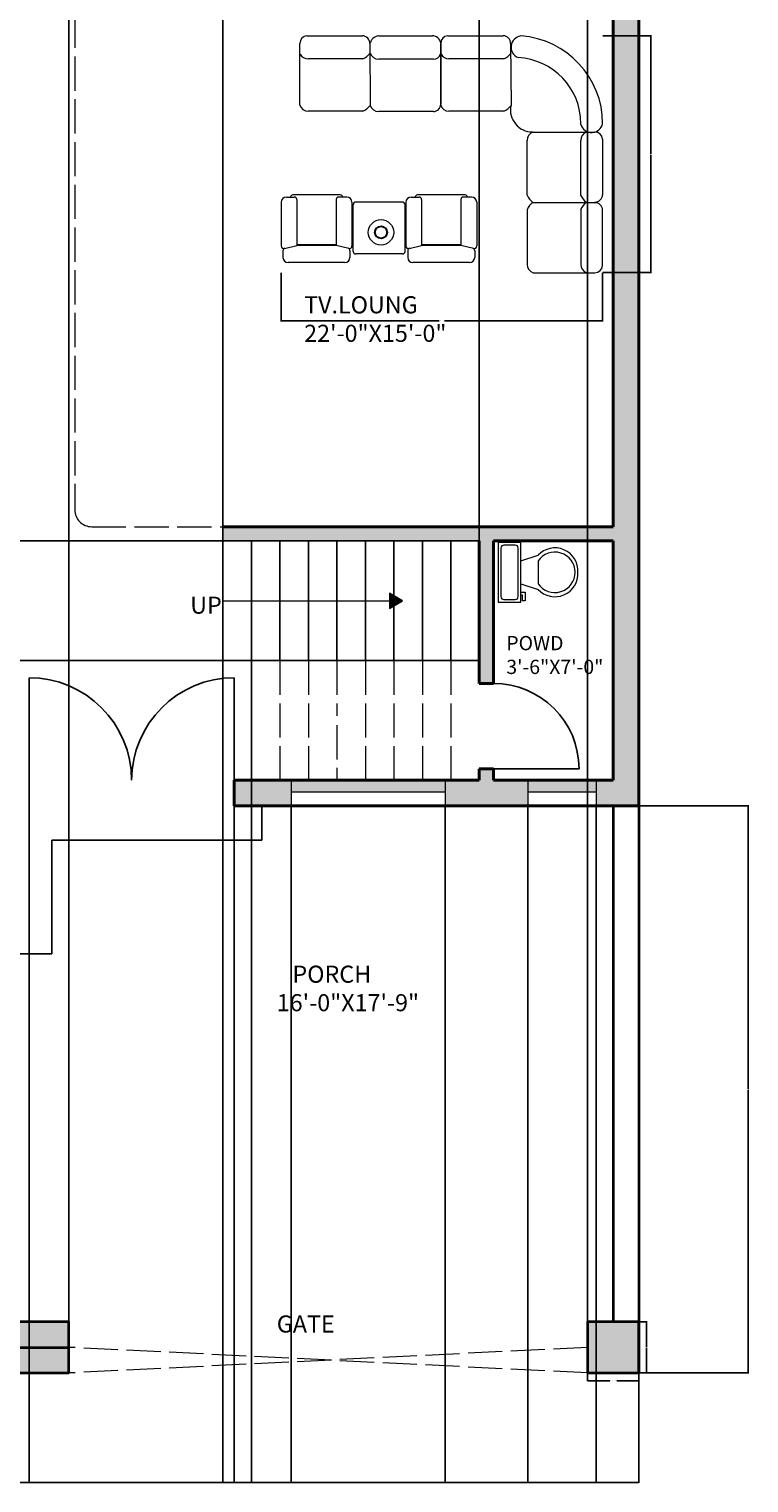
# Model space of a CAD drawing. Units: inches. Extents: x 2985 to 3527, y 3685 to 4528.
# Tile 2 of 5: x 3274 to 3527, y 3685 to 4195. Entities that reach past the tile are written whole.
import ezdxf

# ---------------------------------------------------------------- set-up
doc = ezdxf.new("R2010")
doc.units = ezdxf.units.IN
doc.linetypes.add('ACAD_ISO02W100', pattern=[15, 12, -3])
for name, color, linetype, lineweight in [('A-ANNO-DIMS', 2, 'Continuous', 18), ('A-ANNO-SYMB', 7, 'Continuous', 18), ('A-ANNO-TEXT', 7, 'Continuous', 18), ('A-AREA-IDEN', 7, 'Continuous', 25), ('A-FLOR-EDGE', 7, 'Continuous', 25), ('A-FLOR-FIXT', 9, 'Continuous', 18), ('A-FLOR-STRS', 7, 'Continuous', 25), ('A-FLOR-STRS-OVHD', 7, 'ACAD_ISO02W100', 18), ('A-FURN', 8, 'Continuous', 18), ('A-GLAZ', 4, 'Continuous', 18), ('A-SITE-GATE', 4, 'ACAD_ISO02W100', 18), ('A-SITE-WALL', 7, 'Continuous', 35), ('A-WALL', 7, 'Continuous', 40), ('A-WALL-OVHD', 7, 'ACAD_ISO02W100', 18), ('A-WALL-PATT', 8, 'Continuous', 13), ('door', 4, 'Continuous', 25)]:
    doc.layers.add(name, color=color, linetype=linetype, lineweight=lineweight)
doc.layers.add('A-GLAZ-PATT', color=241, linetype='Continuous', lineweight=13, true_color=0xf7abae)
doc.styles.get("Standard").update_dxf_attribs({"font": 'arial.ttf'})
doc.dimstyles.get("Standard").update_dxf_attribs({"dimtxt": 0.18, "dimasz": 0.18, "dimexe": 0.18, "dimexo": 0.0625, "dimgap": 0.09, "dimtad": 0, "dimtih": 1, "dimtoh": 1, "dimdec": 4, "dimzin": 0, "dimdsep": 46, "dimtxsty": 'Standard', "dimcen": 0.09, "dimadec": 0, "dimazin": 0, "dimtfac": 1, "dimtdec": 4, "dimtofl": 0, "dimtmove": 0, "dimatfit": 3, "dimfxl": 1, "dimtolj": 1, "dimtzin": 0, "dimarcsym": 0})

# ---------------------------------------------------------------- blocks, each defined once
blk = doc.blocks.new('*U7')
for p, q in [((9.5, -6), (9.5, -2)), ((-10, -8.5), (-8, -8.5)), ((-10, -9.5), (-10, -8.5)), ((-7, -9.5), (-10, -9.5)), ((-8, -8.5), (-8, -8)), ((-7, -8), (-7, -9.5)), ((-4, -8), (-6, -14)), ((4, -8), (6, -14)), ((4, -14), (-4, -14))]:
    blk.add_line(p, q)
blk.add_lwpolyline([(10.5, -8), (10.5, 0), (-10.5, 0), (-10.5, -8)], close=True)
for points in [[(-9.5, -2), (-9.5, -6)], [(8.5, -1), (-8.5, -1)], [(-8.5, -7), (8.5, -7)]]:
    blk.add_lwpolyline(points)
for centre, radius, start, end in [((-8.625, -1.875), 0.8839, 81.8699, 188.1301), ((8.625, -1.875), 0.8839, 351.8699, 98.1301), ((-8.625, -6.125), 0.8839, 171.869898, 278.1301), ((8.625, -6.125), 0.8839, 261.8699, 8.1301), ((-0.4772, -19.9188), 8.0953, 133.01722, 273.38), ((0.0374, -19.8731), 7.127, 124.50543, 269.7), ((-0.0373, -19.8731), 7.127, 270.3, 55.4946), ((0.4773, -19.9188), 8.0953, 266.62, 46.9828)]:
    blk.add_arc(centre, radius, start, end)
blk = doc.blocks.new('A$C6748376E')
for p, q in [((297, 2742), (941, 2742)), ((1126, 2742), (1751, 2742)), ((1929, 2742), (2572, 2742)), ((216, 1940), (216, 2654)), ((1026, 2654), (1030, 1936)), ((1847, 2661), (1847, 1951)), ((1847, 1940), (1847, 2654)), ((2657, 2654), (2661, 1936)), ((945, 2475), (312, 2475)), ((1289, 2472), (1130, 2472)), ((1762, 2472), (1289, 2472)), ((2576, 2475), (1943, 2475)), ((945, 1870), (312, 1870)), ((1289, 1866), (1130, 1866)), ((1762, 1866), (1289, 1866)), ((2576, 1870), (1943, 1870)), ((3469, 1717), (3469, 1725)), ((2848, 899), (2848, 1532)), ((2918, 1628), (3632, 1628)), ((3468, 899), (3468, 1532)), ((3538, 1628), (3541, 1628)), ((3721, 1546), (3721, 903)), ((60, 876), (151, 876)), ((684, 900), (136, 900)), ((181, 846), (181, 316)), ((637, 846), (637, 316)), ((760, 876), (667, 876)), ((1504, 876), (1596, 876)), ((2129, 900), (1580, 900)), ((1626, 846), (1626, 316)), ((2081, 846), (2081, 316)), ((2204, 876), (2111, 876)), ((0, 816), (0, 309)), ((820, 816), (820, 309)), ((834, 247), (834, 787)), ((1404, 817), (864, 817)), ((1434, 247), (1434, 787)), ((1444, 816), (1444, 309)), ((2264, 816), (2264, 309)), ((2848, 729), (2848, 96)), ((2915, 814), (3632, 818)), ((2915, 814), (3632, 810)), ((3468, 729), (3468, 96)), ((3721, 81), (3721, 725)), ((21, 253), (21, 246)), ((21, 246), (21, 176)), ((37, 280), (181, 316)), ((637, 324), (181, 324)), ((637, 316), (181, 316)), ((783, 280), (637, 316)), ((797, 253), (797, 176)), ((1404, 217), (864, 217)), ((1466, 253), (1466, 246)), ((1466, 246), (1466, 176)), ((1482, 280), (1626, 316)), ((2081, 324), (1626, 324)), ((2081, 316), (1626, 316)), ((2227, 280), (2081, 316)), ((2241, 253), (2241, 176)), ((737, 116), (81, 116)), ((2181, 116), (1526, 116)), ((2918, 0), (3632, 0)), ((3538, 0), (3541, 0))]:
    blk.add_line(p, q)
for radius in [147, 75, 66]:
    blk.add_circle((1156, 467), radius)
for centre, radius, start, end in [((305, 2654), 89.1, 94.9502, 180), ((941, 2657), 85.2, 357.5912, 90), ((1147, 2618), 126, 99.5063, 163.732), ((1751, 2645), 97.5, 9.5558, 90), ((1936, 2654), 89.1, 94.9502, 180), ((2572, 2657), 85.2, 357.5912, 90), ((2793, 2611), 131, 98.1187, 247.4204), ((2704, 1725), 1018, 0.0517, 86.013), ((312, 2576), 101, 205.9257, 270), ((864, 2667), 208, 292.9498, 323.1162), ((1130, 2578), 106, 199.7589, 270), ((1762, 2557), 85, 269.971, 343.2423), ((1943, 2576), 101, 205.9257, 270), ((2495, 2667), 208, 292.9498, 323.1162), ((2704, 1725), 766, 0, 87.0841), ((312, 1971), 101, 197.7112, 270), ((864, 2061), 208, 292.9498, 323.1162), ((1130, 1972), 106, 199.7589, 270), ((1762, 1951), 85, 269.971, 0), ((1943, 1971), 101, 197.7112, 270), ((2495, 2061), 208, 292.9498, 323.1162), ((2909, 1885), 255, 169.3994, 270), ((3594, 1754), 131, 196.7665, 347.5739), ((2949, 1532), 101, 107.7112, 180), ((3569, 1532), 101, 107.7112, 180), ((3632, 1539), 89.1, 4.9502, 90), ((60, 816), 60, 90, 180), ((136, 870), 30, 90, 180), ((151, 846), 30, 0, 90), ((667, 846), 30, 90, 180), ((684, 870), 30, 0, 90), ((760, 816), 60, 0, 90), ((1504, 816), 60, 90, 180), ((1580, 870), 30, 90, 180), ((1596, 846), 30, 0, 90), ((2111, 846), 30, 90, 180), ((2129, 870), 30, 0, 90), ((2204, 816), 60, 0, 90), ((3039, 980), 208, 202.9498, 233.1162), ((3659, 980), 208, 202.9498, 233.1162), ((3636, 903), 85.2, 267.5912, 0), ((864, 787), 30, 90, 180), ((1404, 787), 30, 0, 90), ((3039, 648), 208, 126.8838, 157.0502), ((3659, 648), 208, 126.8838, 157.0502), ((3636, 725), 85.2, 0, 92.4088), ((30, 309), 30, 180, 284.0362), ((51, 253), 30, 104.0362, 180), ((81, 176), 60, 180, 270), ((737, 176), 60, 270, 0), ((767, 253), 30, 0, 75.9638), ((790, 309), 30, 255.9638, 0), ((864, 247), 30, 180, 270), ((1404, 247), 30, 270, 0), ((1474, 309), 30, 180, 284.0362), ((1496, 253), 30, 104.0362, 180), ((1526, 176), 60, 180, 270), ((2181, 176), 60, 270, 0), ((2211, 253), 30, 0, 75.9638), ((2234, 309), 30, 255.9638, 0), ((2949, 96), 101, 180, 252.2888), ((3569, 96), 101, 180, 252.2888), ((3632, 89), 89.1, 270, 355.0498)]:
    blk.add_arc(centre, radius, start, end)
blk = doc.blocks.new('DOOR-SWING-30IN')
blk.add_line((0, 0), (30, 0))
blk.add_arc((0, 0), 30, 0, 90)
blk = doc.blocks.new('DOOR-SWING-36IN')
blk.add_line((0, 0), (0, 36))
blk.add_arc((0, 0), 36, 0, 90)
blk = doc.blocks.new('GATE-PIER-18IN')
h = blk.add_hatch(color=256)
h.dxf.hatch_style = 1
h.paths.add_polyline_path([(18, 0), (18, 18), (0, 18), (0, 0)])
blk.add_lwpolyline([(0, 0), (18, 0), (18, 18), (0, 18)], close=True)
blk = doc.blocks.new('*D30')
at = {"layer": 'A-ANNO-DIMS', "color": 0, "lineweight": -2, "transparency": 16777216}
for p, q in [((3470.33, 3723.31), (3470.33, 3720.49)), ((3470.51, 3720.67), (3478.1, 3720.67)), ((3488.15, 3720.67), (3480.57, 3720.67)), ((3488.33, 3723.31), (3488.33, 3720.49))]:
    blk.add_line(p, q, dxfattribs=at)
at = {"layer": 'A-ANNO-DIMS', "color": 0, "transparency": 16777216}
for points in [[(3470.51, 3720.7), (3470.51, 3720.64), (3470.33, 3720.67)], [(3488.15, 3720.7), (3488.15, 3720.64), (3488.33, 3720.67)]]:
    blk.add_solid(points, dxfattribs=at)
at = {"layer": 'Defpoints', "color": 0, "transparency": 16777216}
for p in [(3470.33, 3723.37), (3488.33, 3723.37), (3488.33, 3720.67)]:
    blk.add_point(p, dxfattribs=at)
at = {"layer": 'A-ANNO-DIMS', "color": 0, "transparency": 16777216, "insert": (3479.33, 3720.67), "char_height": 0.18, "attachment_point": 5}
blk.add_mtext('\\A1;GATE PIER 18 TYP.', dxfattribs=at)
blk = doc.blocks.new('*D31')
at = {"layer": 'A-ANNO-DIMS', "color": 0, "lineweight": -2, "transparency": 16777216}
for p, q in [((3488.4, 3741.37), (3491.21, 3741.37)), ((3491.03, 3741.19), (3491.03, 3732.55)), ((3491.03, 3723.55), (3491.03, 3732.19)), ((3488.4, 3723.37), (3491.21, 3723.37))]:
    blk.add_line(p, q, dxfattribs=at)
at = {"layer": 'A-ANNO-DIMS', "color": 0, "transparency": 16777216}
for points in [[(3491, 3741.19), (3491.06, 3741.19), (3491.03, 3741.37)], [(3491, 3723.55), (3491.06, 3723.55), (3491.03, 3723.37)]]:
    blk.add_solid(points, dxfattribs=at)
at = {"layer": 'Defpoints', "color": 0, "transparency": 16777216}
for p in [(3488.33, 3741.37), (3491.03, 3741.37), (3488.33, 3723.37)]:
    blk.add_point(p, dxfattribs=at)
at = {"layer": 'A-ANNO-DIMS', "color": 0, "transparency": 16777216, "insert": (3491.03, 3732.37), "char_height": 0.18, "attachment_point": 5}
blk.add_mtext('\\A1;18 TYP.', dxfattribs=at)
blk = doc.blocks.new('*D38')
at = {"layer": 'A-ANNO-DIMS', "color": 0, "lineweight": -2, "transparency": 16777216}
for p, q in [((3362.79, 4109.45), (3362.79, 4092.41)), ((3475.6, 4109.45), (3475.6, 4092.41)), ((3362.97, 4092.59), (3418.25, 4092.59)), ((3475.42, 4092.59), (3420.14, 4092.59))]:
    blk.add_line(p, q, dxfattribs=at)
at = {"layer": 'A-ANNO-DIMS', "color": 0, "transparency": 16777216}
for points in [[(3362.97, 4092.62), (3362.97, 4092.56), (3362.79, 4092.59)], [(3475.42, 4092.62), (3475.42, 4092.56), (3475.6, 4092.59)]]:
    blk.add_solid(points, dxfattribs=at)
at = {"layer": 'Defpoints', "color": 0, "transparency": 16777216}
for p in [(3362.79, 4109.52), (3475.6, 4109.52), (3475.6, 4092.59)]:
    blk.add_point(p, dxfattribs=at)
at = {"layer": 'A-ANNO-DIMS', "color": 0, "transparency": 16777216, "insert": (3419.2, 4092.59), "char_height": 0.18, "attachment_point": 5}
blk.add_mtext('\\A1;SOFA SET 113', dxfattribs=at)
blk = doc.blocks.new('*D39')
at = {"layer": 'A-ANNO-DIMS', "color": 0, "lineweight": -2, "transparency": 16777216}
for p, q in [((3475.66, 4192.64), (3492.7, 4192.64)), ((3492.52, 4192.46), (3492.52, 4151.26)), ((3492.52, 4109.7), (3492.52, 4150.89)), ((3475.66, 4109.52), (3492.7, 4109.52))]:
    blk.add_line(p, q, dxfattribs=at)
at = {"layer": 'A-ANNO-DIMS', "color": 0, "transparency": 16777216}
for points in [[(3492.49, 4192.46), (3492.55, 4192.46), (3492.52, 4192.64)], [(3492.49, 4109.7), (3492.55, 4109.7), (3492.52, 4109.52)]]:
    blk.add_solid(points, dxfattribs=at)
at = {"layer": 'Defpoints', "color": 0, "transparency": 16777216}
for p in [(3475.6, 4192.64), (3492.52, 4192.64), (3475.6, 4109.52)]:
    blk.add_point(p, dxfattribs=at)
at = {"layer": 'A-ANNO-DIMS', "color": 0, "transparency": 16777216, "insert": (3492.52, 4151.08), "char_height": 0.18, "attachment_point": 5}
blk.add_mtext('\\A1;83', dxfattribs=at)
blk = doc.blocks.new('*D40')
at = {"layer": 'A-ANNO-DIMS', "color": 0, "lineweight": -2, "transparency": 16777216}
for p, q in [((3023.83, 3723.31), (3023.83, 3684.79)), ((3488.33, 3723.31), (3488.33, 3684.79)), ((3024.01, 3684.97), (3255.69, 3684.97)), ((3488.15, 3684.97), (3256.48, 3684.97))]:
    blk.add_line(p, q, dxfattribs=at)
at = {"layer": 'A-ANNO-DIMS', "color": 0, "transparency": 16777216}
for points in [[(3024.01, 3685), (3024.01, 3684.94), (3023.83, 3684.97)], [(3488.15, 3685), (3488.15, 3684.94), (3488.33, 3684.97)]]:
    blk.add_solid(points, dxfattribs=at)
at = {"layer": 'Defpoints', "color": 0, "transparency": 16777216}
for p in [(3023.83, 3723.37), (3488.33, 3723.37), (3488.33, 3684.97)]:
    blk.add_point(p, dxfattribs=at)
at = {"layer": 'A-ANNO-DIMS', "color": 0, "transparency": 16777216, "insert": (3256.08, 3684.97), "char_height": 0.18, "attachment_point": 5}
blk.add_mtext('\\A1;464.5', dxfattribs=at)
blk = doc.blocks.new('*D42')
at = {"layer": 'A-ANNO-DIMS', "color": 0, "lineweight": -2, "transparency": 16777216}
for p, q in [((3288.33, 3741.43), (3288.33, 4527.76)), ((3288.51, 4527.58), (3379.05, 4527.58)), ((3470.15, 4527.58), (3379.61, 4527.58)), ((3470.33, 3741.43), (3470.33, 4527.76))]:
    blk.add_line(p, q, dxfattribs=at)
at = {"layer": 'A-ANNO-DIMS', "color": 0, "transparency": 16777216}
for points in [[(3288.51, 4527.61), (3288.51, 4527.55), (3288.33, 4527.58)], [(3470.15, 4527.61), (3470.15, 4527.55), (3470.33, 4527.58)]]:
    blk.add_solid(points, dxfattribs=at)
at = {"layer": 'Defpoints', "color": 0, "transparency": 16777216}
for p in [(3470.33, 4527.58), (3288.33, 3741.37), (3470.33, 3741.37)]:
    blk.add_point(p, dxfattribs=at)
at = {"layer": 'A-ANNO-DIMS', "color": 0, "transparency": 16777216, "insert": (3379.33, 4527.58), "char_height": 0.18, "attachment_point": 5}
blk.add_mtext('\\A1;182', dxfattribs=at)
blk = doc.blocks.new('*D43')
at = {"layer": 'A-ANNO-DIMS', "color": 0, "lineweight": -2, "transparency": 16777216}
for p, q in [((3488.4, 3922.37), (3526.91, 3922.37)), ((3526.73, 3922.19), (3526.73, 3823.05)), ((3526.73, 3723.55), (3526.73, 3822.69)), ((3488.4, 3723.37), (3526.91, 3723.37))]:
    blk.add_line(p, q, dxfattribs=at)
at = {"layer": 'A-ANNO-DIMS', "color": 0, "transparency": 16777216}
for points in [[(3526.7, 3922.19), (3526.76, 3922.19), (3526.73, 3922.37)], [(3526.7, 3723.55), (3526.76, 3723.55), (3526.73, 3723.37)]]:
    blk.add_solid(points, dxfattribs=at)
at = {"layer": 'Defpoints', "color": 0, "transparency": 16777216}
for p in [(3488.33, 3922.37), (3526.73, 3922.37), (3488.33, 3723.37)]:
    blk.add_point(p, dxfattribs=at)
at = {"layer": 'A-ANNO-DIMS', "color": 0, "transparency": 16777216, "insert": (3526.73, 3822.87), "char_height": 0.18, "attachment_point": 5}
blk.add_mtext('\\A1;199', dxfattribs=at)
blk = doc.blocks.new('*D51')
at = {"layer": 'A-ANNO-DIMS', "color": 0, "lineweight": -2, "transparency": 16777216}
for p, q in [((3274.33, 3931.31), (3274.33, 3684.79)), ((3346.33, 3931.31), (3346.33, 3684.79)), ((3274.51, 3684.97), (3310.12, 3684.97)), ((3346.15, 3684.97), (3310.55, 3684.97))]:
    blk.add_line(p, q, dxfattribs=at)
at = {"layer": 'A-ANNO-DIMS', "color": 0, "transparency": 16777216}
for points in [[(3274.51, 3685), (3274.51, 3684.94), (3274.33, 3684.97)], [(3346.15, 3685), (3346.15, 3684.94), (3346.33, 3684.97)]]:
    blk.add_solid(points, dxfattribs=at)
at = {"layer": 'Defpoints', "color": 0, "transparency": 16777216}
for p in [(3274.33, 3931.37), (3346.33, 3931.37), (3346.33, 3684.97)]:
    blk.add_point(p, dxfattribs=at)
at = {"layer": 'A-ANNO-DIMS', "color": 0, "transparency": 16777216, "insert": (3310.33, 3684.97), "char_height": 0.18, "attachment_point": 5}
blk.add_mtext('\\A1;72', dxfattribs=at)
blk = doc.blocks.new('*D52')
at = {"layer": 'A-ANNO-DIMS', "color": 0, "lineweight": -2, "transparency": 16777216}
for p, q in [((3342.27, 4015.37), (2985.25, 4015.37)), ((2985.43, 4015.19), (2985.43, 3994.55)), ((2985.43, 3973.55), (2985.43, 3994.19)), ((3342.27, 3973.37), (2985.25, 3973.37))]:
    blk.add_line(p, q, dxfattribs=at)
at = {"layer": 'A-ANNO-DIMS', "color": 0, "transparency": 16777216}
for points in [[(2985.4, 4015.19), (2985.46, 4015.19), (2985.43, 4015.37)], [(2985.4, 3973.55), (2985.46, 3973.55), (2985.43, 3973.37)]]:
    blk.add_solid(points, dxfattribs=at)
at = {"layer": 'Defpoints', "color": 0, "transparency": 16777216}
for p in [(2985.43, 4015.37), (3342.33, 4015.37), (3342.33, 3973.37)]:
    blk.add_point(p, dxfattribs=at)
at = {"layer": 'A-ANNO-DIMS', "color": 0, "transparency": 16777216, "insert": (2985.43, 3994.37), "char_height": 0.18, "attachment_point": 5}
blk.add_mtext('\\A1;42', dxfattribs=at)
blk = doc.blocks.new('*D53')
at = {"layer": 'A-ANNO-DIMS', "color": 0, "lineweight": -2, "transparency": 16777216}
for p, q in [((3342.33, 4015.43), (3342.33, 4527.76)), ((3342.51, 4527.58), (3387.11, 4527.58)), ((3432.15, 4527.58), (3387.55, 4527.58)), ((3432.33, 4015.43), (3432.33, 4527.76))]:
    blk.add_line(p, q, dxfattribs=at)
at = {"layer": 'A-ANNO-DIMS', "color": 0, "transparency": 16777216}
for points in [[(3342.51, 4527.61), (3342.51, 4527.55), (3342.33, 4527.58)], [(3432.15, 4527.61), (3432.15, 4527.55), (3432.33, 4527.58)]]:
    blk.add_solid(points, dxfattribs=at)
at = {"layer": 'Defpoints', "color": 0, "transparency": 16777216}
for p in [(3432.33, 4527.58), (3342.33, 4015.37), (3432.33, 4015.37)]:
    blk.add_point(p, dxfattribs=at)
at = {"layer": 'A-ANNO-DIMS', "color": 0, "transparency": 16777216, "insert": (3387.33, 4527.58), "char_height": 0.18, "attachment_point": 5}
blk.add_mtext('\\A1;90', dxfattribs=at)
blk = doc.blocks.new('*D54')
at = {"layer": 'A-ANNO-DIMS', "color": 0, "lineweight": -2, "transparency": 16777216}
for p, q in [((3342.33, 3973.31), (3342.33, 3684.79)), ((3352.33, 3973.31), (3352.33, 3684.79)), ((3342.51, 3684.97), (3347.12, 3684.97)), ((3352.15, 3684.97), (3347.54, 3684.97))]:
    blk.add_line(p, q, dxfattribs=at)
at = {"layer": 'A-ANNO-DIMS', "color": 0, "transparency": 16777216}
for points in [[(3342.51, 3685), (3342.51, 3684.94), (3342.33, 3684.97)], [(3352.15, 3685), (3352.15, 3684.94), (3352.33, 3684.97)]]:
    blk.add_solid(points, dxfattribs=at)
at = {"layer": 'Defpoints', "color": 0, "transparency": 16777216}
for p in [(3342.33, 3973.37), (3352.33, 3973.37), (3352.33, 3684.97)]:
    blk.add_point(p, dxfattribs=at)
at = {"layer": 'A-ANNO-DIMS', "color": 0, "transparency": 16777216, "insert": (3347.33, 3684.97), "char_height": 0.18, "attachment_point": 5}
blk.add_mtext('\\A1;10', dxfattribs=at)
blk = doc.blocks.new('*D55')
at = {"layer": 'A-ANNO-DIMS', "color": 0, "lineweight": -2, "transparency": 16777216}
for p, q in [((3366.33, 3922.31), (3366.33, 3684.79)), ((3420.33, 3922.31), (3420.33, 3684.79)), ((3366.51, 3684.97), (3393.11, 3684.97)), ((3420.15, 3684.97), (3393.55, 3684.97))]:
    blk.add_line(p, q, dxfattribs=at)
at = {"layer": 'A-ANNO-DIMS', "color": 0, "transparency": 16777216}
for points in [[(3366.51, 3685), (3366.51, 3684.94), (3366.33, 3684.97)], [(3420.15, 3685), (3420.15, 3684.94), (3420.33, 3684.97)]]:
    blk.add_solid(points, dxfattribs=at)
at = {"layer": 'Defpoints', "color": 0, "transparency": 16777216}
for p in [(3366.33, 3922.37), (3420.33, 3922.37), (3420.33, 3684.97)]:
    blk.add_point(p, dxfattribs=at)
at = {"layer": 'A-ANNO-DIMS', "color": 0, "transparency": 16777216, "insert": (3393.33, 3684.97), "char_height": 0.18, "attachment_point": 5}
blk.add_mtext('\\A1;54', dxfattribs=at)
blk = doc.blocks.new('*D56')
at = {"layer": 'A-ANNO-DIMS', "color": 0, "lineweight": -2, "transparency": 16777216}
for p, q in [((3449.33, 3922.31), (3449.33, 3684.79)), ((3473.33, 3922.31), (3473.33, 3684.79)), ((3449.51, 3684.97), (3461.11, 3684.97)), ((3473.15, 3684.97), (3461.55, 3684.97))]:
    blk.add_line(p, q, dxfattribs=at)
at = {"layer": 'A-ANNO-DIMS', "color": 0, "transparency": 16777216}
for points in [[(3449.51, 3685), (3449.51, 3684.94), (3449.33, 3684.97)], [(3473.15, 3685), (3473.15, 3684.94), (3473.33, 3684.97)]]:
    blk.add_solid(points, dxfattribs=at)
at = {"layer": 'Defpoints', "color": 0, "transparency": 16777216}
for p in [(3449.33, 3922.37), (3473.33, 3922.37), (3473.33, 3684.97)]:
    blk.add_point(p, dxfattribs=at)
at = {"layer": 'A-ANNO-DIMS', "color": 0, "transparency": 16777216, "insert": (3461.33, 3684.97), "char_height": 0.18, "attachment_point": 5}
blk.add_mtext('\\A1;24', dxfattribs=at)
blk = doc.blocks.new('*D60')
at = {"layer": 'A-ANNO-DIMS', "color": 0, "lineweight": -2, "transparency": 16777216}
for p, q in [((3346.33, 3922.31), (3346.33, 3684.79)), ((3366.33, 3922.31), (3366.33, 3684.79)), ((3346.51, 3684.97), (3356.11, 3684.97)), ((3366.15, 3684.97), (3356.55, 3684.97))]:
    blk.add_line(p, q, dxfattribs=at)
at = {"layer": 'A-ANNO-DIMS', "color": 0, "transparency": 16777216}
for points in [[(3346.51, 3685), (3346.51, 3684.94), (3346.33, 3684.97)], [(3366.15, 3685), (3366.15, 3684.94), (3366.33, 3684.97)]]:
    blk.add_solid(points, dxfattribs=at)
at = {"layer": 'Defpoints', "color": 0, "transparency": 16777216}
for p in [(3346.33, 3922.37), (3366.33, 3922.37), (3366.33, 3684.97)]:
    blk.add_point(p, dxfattribs=at)
at = {"layer": 'A-ANNO-DIMS', "color": 0, "transparency": 16777216, "insert": (3356.33, 3684.97), "char_height": 0.18, "attachment_point": 5}
blk.add_mtext('\\A1;20', dxfattribs=at)
blk = doc.blocks.new('*D61')
at = {"layer": 'A-ANNO-DIMS', "color": 0, "lineweight": -2, "transparency": 16777216}
for p, q in [((3473.33, 3922.31), (3473.33, 3684.79)), ((3488.33, 3922.31), (3488.33, 3684.79)), ((3473.51, 3684.97), (3480.62, 3684.97)), ((3488.15, 3684.97), (3481.04, 3684.97))]:
    blk.add_line(p, q, dxfattribs=at)
at = {"layer": 'A-ANNO-DIMS', "color": 0, "transparency": 16777216}
for points in [[(3473.51, 3685), (3473.51, 3684.94), (3473.33, 3684.97)], [(3488.15, 3685), (3488.15, 3684.94), (3488.33, 3684.97)]]:
    blk.add_solid(points, dxfattribs=at)
at = {"layer": 'Defpoints', "color": 0, "transparency": 16777216}
for p in [(3473.33, 3922.37), (3488.33, 3922.37), (3488.33, 3684.97)]:
    blk.add_point(p, dxfattribs=at)
at = {"layer": 'A-ANNO-DIMS', "color": 0, "transparency": 16777216, "insert": (3480.83, 3684.97), "char_height": 0.18, "attachment_point": 5}
blk.add_mtext('\\A1;15', dxfattribs=at)

msp = doc.modelspace()

# ---------------------------------------------------------------- hatches: boundary and pattern name
at = {"layer": 'A-ANNO-SYMB'}
h = msp.add_hatch(color=256, dxfattribs=at)
h.dxf.hatch_style = 1
h.paths.add_polyline_path([(3405.403, 3994.372), (3400.799, 3997.03), (3400.799, 3991.713)])
at = {"layer": 'A-GLAZ-PATT'}
h = msp.add_hatch(color=256, dxfattribs=at)
h.dxf.hatch_style = 1
h.paths.add_polyline_path([(3420.333, 3931.372), (3366.333, 3931.372), (3366.333, 3927.372), (3420.333, 3927.372)])
h = msp.add_hatch(color=256, dxfattribs=at)
h.dxf.hatch_style = 1
h.paths.add_polyline_path([(3473.333, 3931.372), (3449.333, 3931.372), (3449.333, 3927.372), (3473.333, 3927.372)])
at = {"layer": 'A-WALL-PATT'}
h = msp.add_hatch(color=256, dxfattribs=at)
h.dxf.hatch_style = 1
h.paths.add_polyline_path([(3488.333, 4439.372), (3319.833, 4439.372), (3319.833, 4430.372), (3367.833, 4430.372), (3367.833, 4404.372), (3372.833, 4404.372), (3372.833, 4430.372), (3479.333, 4430.372), (3479.333, 4370.372), (3453.333, 4370.372), (3445.333, 4370.372), (3445.333, 4365.372), (3479.333, 4365.372), (3479.333, 4209.372), (3299.333, 4209.372), (3299.333, 4213.372), (3290.333, 4213.372), (3290.333, 4200.372), (3479.333, 4200.372), (3479.333, 4020.372), (3342.333, 4020.372), (3342.333, 4015.372), (3432.333, 4015.372), (3432.333, 3965.372), (3437.333, 3965.372), (3437.333, 4015.372), (3479.333, 4015.372), (3479.333, 3931.372), (3473.333, 3931.372), (3473.333, 3922.372), (3488.333, 3922.372)])
h = msp.add_hatch(color=256, dxfattribs=at)
h.dxf.hatch_style = 1
h.paths.add_polyline_path([(3449.333, 3931.372), (3437.333, 3931.372), (3437.333, 3935.372), (3432.333, 3935.372), (3432.333, 3931.372), (3420.333, 3931.372), (3420.333, 3922.372), (3449.333, 3922.372)])
h = msp.add_hatch(color=256, dxfattribs=at)
h.dxf.hatch_style = 1
h.paths.add_polyline_path([(3366.333, 3931.372), (3346.333, 3931.372), (3346.333, 3922.372), (3366.333, 3922.372)])

# ---------------------------------------------------------------- linework, layer by layer
at = {"layer": 'A-ANNO-SYMB'}
msp.add_line((3342.333, 3994.372), (3400.799, 3994.372), dxfattribs=at)
msp.add_lwpolyline([(3405.403, 3994.372), (3400.799, 3997.03), (3400.799, 3991.713)], close=True, dxfattribs=at)
at = {"layer": 'A-FLOR-EDGE'}
for p, q in [((3355.964, 3922.372), (3355.964, 3910.372)), ((3355.964, 3910.372), (3282.333, 3910.372)), ((3282.333, 3870.449), (3282.333, 3910.372)), ((3270.333, 3870.449), (3282.333, 3870.449))]:
    msp.add_line(p, q, dxfattribs=at)
at = {"layer": 'A-FLOR-STRS'}
for p, q in [((3342.333, 4020.372), (3342.333, 3973.372)), ((3342.333, 4015.372), (3432.333, 4015.372)), ((3352.333, 4015.372), (3352.333, 3973.372)), ((3362.333, 4015.372), (3362.333, 3973.372)), ((3372.333, 4015.372), (3372.333, 3973.372)), ((3382.333, 4015.372), (3382.333, 3973.372)), ((3392.333, 4015.372), (3392.333, 3973.372)), ((3402.333, 4015.372), (3402.333, 3996.144)), ((3412.333, 4015.372), (3412.333, 3973.372)), ((3422.333, 4015.372), (3422.333, 3973.372)), ((3402.333, 3992.6), (3402.333, 3973.372)), ((3342.333, 3973.372), (3432.333, 3973.372))]:
    msp.add_line(p, q, dxfattribs=at)
at = {"layer": 'A-FLOR-STRS-OVHD'}
for p, q in [((3352.333, 3973.372), (3352.333, 3931.372)), ((3362.333, 3973.372), (3362.333, 3931.372)), ((3372.333, 3973.372), (3372.333, 3931.372)), ((3382.333, 3973.372), (3382.333, 3954.016)), ((3392.333, 3973.372), (3392.333, 3931.372)), ((3402.333, 3973.372), (3402.333, 3931.372)), ((3412.333, 3973.372), (3412.333, 3931.372)), ((3422.333, 3973.372), (3422.333, 3931.372)), ((3382.333, 3950.728), (3382.333, 3931.372))]:
    msp.add_line(p, q, dxfattribs=at)
at = {"layer": 'A-GLAZ'}
for p, q in [((3366.333, 3931.372), (3366.333, 3922.372)), ((3420.333, 3931.372), (3420.333, 3922.372)), ((3449.333, 3931.372), (3449.333, 3922.372)), ((3473.333, 3931.372), (3473.333, 3922.372)), ((3366.333, 3927.372), (3420.333, 3927.372)), ((3449.333, 3927.372), (3473.333, 3927.372))]:
    msp.add_line(p, q, dxfattribs=at)
at = {"layer": 'A-SITE-GATE'}
for p, q in [((3470.333, 3732.372), (3288.333, 3723.372)), ((3470.333, 3723.372), (3288.333, 3732.372))]:
    msp.add_line(p, q, dxfattribs=at)
at = {"layer": 'A-SITE-WALL'}
for p, q in [((3479.333, 3922.372), (3479.333, 3741.372)), ((3488.333, 3922.372), (3488.333, 3723.372)), ((3032.833, 3732.372), (3288.333, 3732.372)), ((3023.833, 3723.372), (3288.333, 3723.372))]:
    msp.add_line(p, q, dxfattribs=at)
at = {"layer": 'A-WALL'}
for p, q in [((3488.333, 4439.372), (3488.333, 3922.372)), ((3479.333, 4200.372), (3479.333, 4020.372)), ((3342.333, 4020.372), (3479.333, 4020.372)), ((3432.333, 4015.372), (3432.333, 3965.372)), ((3437.333, 4015.372), (3437.333, 3965.372)), ((3437.333, 4015.372), (3479.333, 4015.372)), ((3479.333, 4015.372), (3479.333, 3931.372)), ((3432.333, 3965.372), (3437.333, 3965.372)), ((3432.333, 3935.372), (3437.333, 3935.372)), ((3432.333, 3935.372), (3432.333, 3931.372)), ((3437.333, 3935.372), (3437.333, 3931.372)), ((3346.333, 3931.372), (3346.333, 3922.372)), ((3346.333, 3931.372), (3432.333, 3931.372)), ((3437.333, 3931.372), (3479.333, 3931.372)), ((3346.333, 3922.372), (3488.333, 3922.372))]:
    msp.add_line(p, q, dxfattribs=at)
at = {"layer": 'A-WALL-OVHD'}
for p, q in [((3290.333, 4200.372), (3290.333, 4026.372)), ((3296.333, 4020.372), (3342.333, 4020.372))]:
    msp.add_line(p, q, dxfattribs=at)
msp.add_arc((3296.333, 4026.372), 6, 180, 270, dxfattribs=at)

# ---------------------------------------------------------------- block references
at = {"layer": 'A-FLOR-FIXT', "rotation": 90}
msp.add_blockref('*U7', (3438.936, 4004.359), dxfattribs=at)
at = {"layer": 'A-FURN', "xscale": 0.0303106538473338, "yscale": 0.0303106538473338, "zscale": 0.0303106538473338}
msp.add_blockref('A$C6748376E', (3362.791, 4109.515), dxfattribs=at)
at = {"layer": 'A-SITE-WALL'}
for p in [(3270.333, 3723.372), (3470.333, 3723.372)]:
    msp.add_blockref('GATE-PIER-18IN', p, dxfattribs=at)
at = {"layer": 'door'}
for name, p in [('DOOR-SWING-36IN', (3274.333, 3931.372)), ('DOOR-SWING-30IN', (3437.333, 3935.372))]:
    msp.add_blockref(name, p, dxfattribs=at)
at = {"layer": 'door', "extrusion": (0, 0, -1), "zscale": -1}
msp.add_blockref('DOOR-SWING-36IN', (-3346.333, 3931.372), dxfattribs=at)

# ---------------------------------------------------------------- texts
at = {"layer": 'A-ANNO-TEXT', "char_height": 6, "attachment_point": 1}
for s, width, insert in [('UP ', 25.1087, (3330.871, 3995.823)), ('GATE', 91.11669, (3361.249, 3743.568))]:
    msp.add_mtext_dynamic_manual_height_columns(s, width=width, gutter_width=12.5, heights=[0], dxfattribs=dict(at, insert=insert))
at = {"layer": 'A-AREA-IDEN', "attachment_point": 1}
for s, width, insert, char_height in [('TV.LOUNG\\P22\'-0"X15\'-0"', 94.1084, (3370.859, 4101.241), 6), ('POWD\\P3\'-6"X7\'-0"', 20.83824, (3441.807, 3982.009), 5), ('   PORCH\\P16\'-0"X17\'-9"', 91.11669, (3361.249, 3866.328), 6)]:
    msp.add_mtext_dynamic_manual_height_columns(s, width=width, gutter_width=12.5, heights=[0], dxfattribs=dict(at, insert=insert, char_height=char_height))

# ---------------------------------------------------------------- dimensions: what is measured, and where the dimension line sits
at = {"layer": 'A-ANNO-DIMS'}
for base, p1, p2, override, picture, middle in [((3470.333, 4527.583), (3288.333, 3741.372), (3470.333, 3741.372), {"dimdec": 0, "dimlfac": 1, "dimrnd": 0, "dimzin": 0, "dimdsep": 46, "dimlunit": 2}, '*D42', (3379.333, 4527.583)), ((3432.333, 4527.583), (3342.333, 4015.372), (3432.333, 4015.372), {"dimdec": 0, "dimlfac": 1, "dimrnd": 0, "dimzin": 0, "dimdsep": 46, "dimlunit": 2}, '*D53', (3387.333, 4527.583)), ((3352.333, 3684.972), (3342.333, 3973.372), (3352.333, 3973.372), {"dimdec": 0, "dimlfac": 1, "dimrnd": 0, "dimzin": 0, "dimdsep": 46, "dimlunit": 2}, '*D54', (3347.333, 3684.972)), ((3346.333, 3684.972), (3274.333, 3931.372), (3346.333, 3931.372), {"dimdec": 0, "dimlfac": 1, "dimrnd": 0, "dimzin": 0, "dimdsep": 46, "dimlunit": 2}, '*D51', (3310.333, 3684.972)), ((3366.333, 3684.972), (3346.333, 3922.372), (3366.333, 3922.372), {"dimdec": 0, "dimlfac": 1, "dimrnd": 0, "dimzin": 0, "dimdsep": 46, "dimlunit": 2}, '*D60', (3356.333, 3684.972)), ((3420.333, 3684.972), (3366.333, 3922.372), (3420.333, 3922.372), {"dimdec": 0, "dimlfac": 1, "dimrnd": 0, "dimzin": 0, "dimdsep": 46, "dimlunit": 2}, '*D55', (3393.333, 3684.972)), ((3473.333, 3684.972), (3449.333, 3922.372), (3473.333, 3922.372), {"dimdec": 0, "dimlfac": 1, "dimrnd": 0, "dimzin": 0, "dimdsep": 46, "dimlunit": 2}, '*D56', (3461.333, 3684.972)), ((3488.333, 3684.972), (3473.333, 3922.372), (3488.333, 3922.372), {"dimdec": 0, "dimlfac": 1, "dimrnd": 0, "dimzin": 0, "dimdsep": 46, "dimlunit": 2}, '*D61', (3480.833, 3684.972)), ((3488.333, 3684.972), (3023.833, 3723.372), (3488.333, 3723.372), {"dimdec": 1, "dimlfac": 1, "dimrnd": 0, "dimzin": 0, "dimdsep": 46, "dimlunit": 2}, '*D40', (3256.083, 3684.972))]:
    dim = msp.add_linear_dim(base=base, p1=p1, p2=p2, dimstyle='Standard', override=override, dxfattribs=at)
    dim.commit()
    dim.dimension.update_dxf_attribs({"geometry": picture, "text_midpoint": middle})
for base, p1, p2, picture, middle in [((3492.523, 4192.637), (3475.602, 4109.515), (3475.602, 4192.637), '*D39', (3492.523, 4151.076)), ((2985.433, 4015.372), (3342.333, 3973.372), (3342.333, 4015.372), '*D52', (2985.433, 3994.372)), ((3526.733, 3922.372), (3488.333, 3723.372), (3488.333, 3922.372), '*D43', (3526.733, 3822.872))]:
    dim = msp.add_linear_dim(base=base, p1=p1, p2=p2, angle=90, dimstyle='Standard', override={"dimdec": 0, "dimlfac": 1, "dimrnd": 0, "dimzin": 0, "dimdsep": 46, "dimlunit": 2}, dxfattribs=at)
    dim.commit()
    dim.dimension.update_dxf_attribs({"geometry": picture, "text_midpoint": middle})
for base, p1, p2, text, picture, middle in [((3475.602, 4092.594), (3362.791, 4109.515), (3475.602, 4109.515), 'SOFA SET <>', '*D38', (3419.196, 4092.594)), ((3488.333, 3720.672), (3470.333, 3723.372), (3488.333, 3723.372), 'GATE PIER <> TYP.', '*D30', (3479.333, 3720.672))]:
    dim = msp.add_linear_dim(base=base, p1=p1, p2=p2, text=text, dimstyle='Standard', override={"dimdec": 0, "dimlfac": 1, "dimrnd": 0, "dimzin": 0, "dimdsep": 46, "dimlunit": 2}, dxfattribs=at)
    dim.commit()
    dim.dimension.update_dxf_attribs({"geometry": picture, "text_midpoint": middle})
dim = msp.add_linear_dim(base=(3491.033, 3741.372), p1=(3488.333, 3723.372), p2=(3488.333, 3741.372), angle=90, text='<> TYP.', dimstyle='Standard', override={"dimdec": 0, "dimlfac": 1, "dimrnd": 0, "dimzin": 0, "dimdsep": 46, "dimlunit": 2}, dxfattribs=at)
dim.commit()
dim.dimension.update_dxf_attribs({"geometry": '*D31', "text_midpoint": (3491.033, 3732.372)})

doc.saveas('drawing.dxf')
